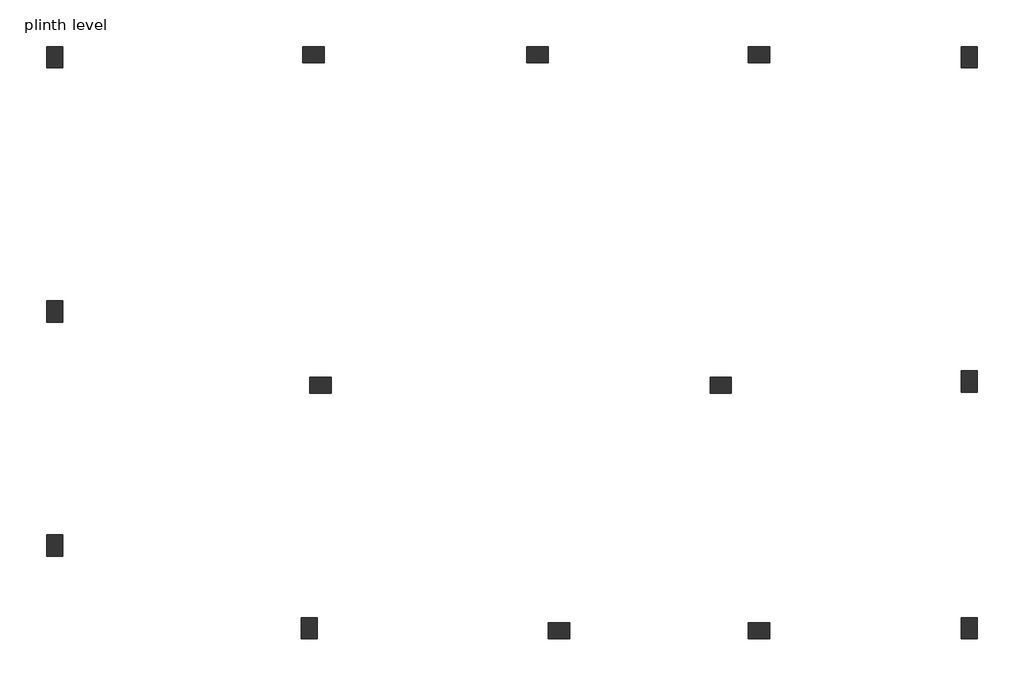
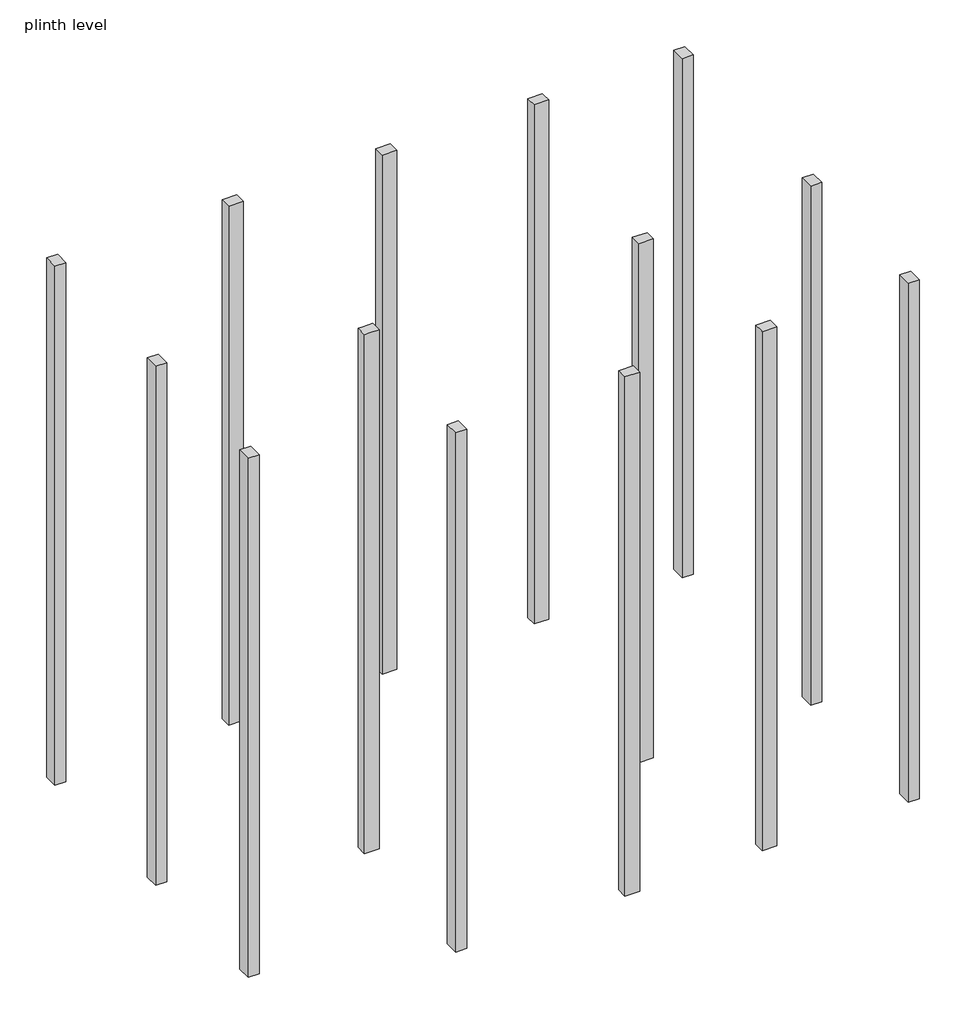
# One storey: 14 columns.
"""IFC4 building model written with IfcOpenShell, lengths in millimetres."""

from ifc_helpers import new_model, si_unit, origin, place, context, project, spatial, faceted_brep, element, save

model = new_model("IFC4")

# Units and contexts
model_context = context("Model", 3, world=origin())
ifc_project = project(units=[si_unit("LENGTHUNIT", "METRE", prefix="MILLI")], contexts=[model_context])

# Site, building, storey
site = spatial("IfcSite", under=ifc_project)
building = spatial("IfcBuilding", under=site)
storey = spatial("IfcBuildingStorey", under=building, Name="plinth level", Elevation=-1219.2)

# Columns
placement = place(None, origin())
element("IfcColumn", 1, ObjectType="Concrete-Rectangular-Column", at=placement, inside=storey, context=model_context, shape_type="Brep", body=[
    faceted_brep([(-8931.9263529, 6682.6661978, -1219.2), (-8931.9263529, 6377.8661978, -1219.2), (-9160.5263529, 6377.8661978, -1219.2), (-9160.5263529, 6682.6661978, -1219.2), (-8931.9263529, 6682.6661978, 10210.8), (-8931.9263529, 6377.8661978, 10210.8), (-8931.9263529, 6377.8661978, 9906.0), (-8931.9263529, 6377.8661978, 7010.4), (-8931.9263529, 6377.8661978, 6705.6), (-8931.9263529, 6377.8661978, 3810.0), (-8931.9263529, 6377.8661978, 3505.2), (-8931.9263529, 6377.8661978, 609.6), (-8931.9263529, 6377.8661978, 304.8), (-8931.9263529, 6682.6661978, 304.8), (-8931.9263529, 6682.6661978, 609.6), (-8931.9263529, 6682.6661978, 3505.2), (-8931.9263529, 6682.6661978, 3810.0), (-8931.9263529, 6682.6661978, 6705.6), (-8931.9263529, 6682.6661978, 7010.4), (-8931.9263529, 6682.6661978, 9906.0), (-9160.5263529, 6377.8661978, 10210.8), (-9160.5263529, 6377.8661978, 9906.0), (-9160.5263529, 6377.8661978, 7010.4), (-9160.5263529, 6377.8661978, 6705.6), (-9160.5263529, 6377.8661978, 3810.0), (-9160.5263529, 6377.8661978, 3505.2), (-9160.5263529, 6377.8661978, 609.6), (-9160.5263529, 6377.8661978, 304.8), (-9160.5263529, 6682.6661978, 10210.8), (-9160.5263529, 6682.6661978, 9906.0), (-9160.5263529, 6682.6661978, 7010.4), (-9160.5263529, 6682.6661978, 6705.6), (-9160.5263529, 6682.6661978, 3810.0), (-9160.5263529, 6682.6661978, 3505.2), (-9160.5263529, 6682.6661978, 609.6), (-9160.5263529, 6682.6661978, 304.8)], [[[0, 1, 2, 3]], [[4, 5, 6, 7, 8, 9, 10, 11, 12, 1, 0, 13, 14, 15, 16, 17, 18, 19]], [[5, 20, 21, 22, 23, 24, 25, 26, 27, 2, 1, 12, 11, 10, 9, 8, 7, 6]], [[20, 28, 29, 30, 31, 32, 33, 34, 35, 3, 2, 27, 26, 25, 24, 23, 22, 21]], [[28, 4, 19, 18, 17, 16, 15, 14, 13, 0, 3, 35, 34, 33, 32, 31, 30, 29]], [[4, 28, 20, 5]]]),
])
element("IfcColumn", 2, ObjectType="Concrete-Rectangular-Column", at=placement, inside=storey, context=model_context, shape_type="Brep", body=[
    faceted_brep([(-5502.9263529, 6682.6661978, -1219.2), (-5198.1263529, 6682.6661978, -1219.2), (-5198.1263529, 6454.0661978, -1219.2), (-5502.9263529, 6454.0661978, -1219.2), (-5502.9263529, 6682.6661978, 10210.8), (-5198.1263529, 6682.6661978, 10210.8), (-5198.1263529, 6644.5661978, 10210.8), (-5198.1263529, 6454.0661978, 10210.8), (-5198.1263529, 6454.0661978, 9906.0), (-5198.1263529, 6454.0661978, 7010.4), (-5198.1263529, 6454.0661978, 6705.6), (-5198.1263529, 6454.0661978, 3810.0), (-5198.1263529, 6454.0661978, 3505.2), (-5198.1263529, 6454.0661978, 609.6), (-5198.1263529, 6454.0661978, 304.8), (-5502.9263529, 6454.0661978, 10210.8), (-5502.9263529, 6454.0661978, 9906.0), (-5502.9263529, 6454.0661978, 7010.4), (-5502.9263529, 6454.0661978, 6705.6), (-5502.9263529, 6454.0661978, 3810.0), (-5502.9263529, 6454.0661978, 3505.2), (-5502.9263529, 6454.0661978, 609.6), (-5502.9263529, 6454.0661978, 304.8), (-5502.9263529, 6644.5661978, 10210.8)], [[[0, 1, 2, 3]], [[4, 5, 1, 0]], [[5, 6, 7, 8, 9, 10, 11, 12, 13, 14, 2, 1]], [[7, 15, 16, 17, 18, 19, 20, 21, 22, 3, 2, 14, 13, 12, 11, 10, 9, 8]], [[15, 23, 4, 0, 3, 22, 21, 20, 19, 18, 17, 16]], [[4, 23, 15, 7, 6, 5]]]),
])
element("IfcColumn", 3, ObjectType="Concrete-Rectangular-Column", at=placement, inside=storey, context=model_context, shape_type="Brep", body=[
    faceted_brep([(-2302.5263529, 6682.6661978, -1219.2), (-1997.7263529, 6682.6661978, -1219.2), (-1997.7263529, 6454.0661978, -1219.2), (-2302.5263529, 6454.0661978, -1219.2), (-2302.5263529, 6682.6661978, 10210.8), (-1997.7263529, 6682.6661978, 10210.8), (-1997.7263529, 6644.5661978, 10210.8), (-1997.7263529, 6454.0661978, 10210.8), (-1997.7263529, 6454.0661978, 9906.0), (-1997.7263529, 6454.0661978, 7010.4), (-1997.7263529, 6454.0661978, 6705.6), (-1997.7263529, 6454.0661978, 3810.0), (-1997.7263529, 6454.0661978, 3505.2), (-1997.7263529, 6454.0661978, 609.6), (-1997.7263529, 6454.0661978, 304.8), (-2302.5263529, 6454.0661978, 10210.8), (-2302.5263529, 6454.0661978, 9906.0), (-2302.5263529, 6454.0661978, 7010.4), (-2302.5263529, 6454.0661978, 6705.6), (-2302.5263529, 6454.0661978, 3810.0), (-2302.5263529, 6454.0661978, 3505.2), (-2302.5263529, 6454.0661978, 609.6), (-2302.5263529, 6454.0661978, 304.8), (-2302.5263529, 6644.5661978, 10210.8)], [[[0, 1, 2, 3]], [[4, 5, 1, 0]], [[5, 6, 7, 8, 9, 10, 11, 12, 13, 14, 2, 1]], [[7, 15, 16, 17, 18, 19, 20, 21, 22, 3, 2, 14, 13, 12, 11, 10, 9, 8]], [[15, 23, 4, 0, 3, 22, 21, 20, 19, 18, 17, 16]], [[4, 23, 15, 7, 6, 5]]]),
])
element("IfcColumn", 4, ObjectType="Concrete-Rectangular-Column", at=placement, inside=storey, context=model_context, shape_type="Brep", body=[
    faceted_brep([(859.7736471, 6682.6661978, -1219.2), (1164.5736471, 6682.6661978, -1219.2), (1164.5736471, 6454.0661978, -1219.2), (859.7736471, 6454.0661978, -1219.2), (859.7736471, 6682.6661978, 10210.8), (1164.5736471, 6682.6661978, 10210.8), (1164.5736471, 6644.5661978, 10210.8), (1164.5736471, 6454.0661978, 10210.8), (1164.5736471, 6454.0661978, 9906.0), (1164.5736471, 6454.0661978, 7010.4), (1164.5736471, 6454.0661978, 6705.6), (1164.5736471, 6454.0661978, 3810.0), (1164.5736471, 6454.0661978, 3505.2), (1164.5736471, 6454.0661978, 609.6), (1164.5736471, 6454.0661978, 304.8), (859.7736471, 6454.0661978, 10210.8), (859.7736471, 6454.0661978, 9906.0), (859.7736471, 6454.0661978, 7010.4), (859.7736471, 6454.0661978, 6705.6), (859.7736471, 6454.0661978, 3810.0), (859.7736471, 6454.0661978, 3505.2), (859.7736471, 6454.0661978, 609.6), (859.7736471, 6454.0661978, 304.8), (859.7736471, 6644.5661978, 10210.8)], [[[0, 1, 2, 3]], [[4, 5, 1, 0]], [[5, 6, 7, 8, 9, 10, 11, 12, 13, 14, 2, 1]], [[7, 15, 16, 17, 18, 19, 20, 21, 22, 3, 2, 14, 13, 12, 11, 10, 9, 8]], [[15, 23, 4, 0, 3, 22, 21, 20, 19, 18, 17, 16]], [[4, 23, 15, 7, 6, 5]]]),
])
element("IfcColumn", 5, ObjectType="Concrete-Rectangular-Column", at=placement, inside=storey, context=model_context, shape_type="Brep", body=[
    faceted_brep([(3901.4236471, 6377.8661978, -1219.2), (3901.4236471, 6682.6661978, -1219.2), (4130.0236471, 6682.6661978, -1219.2), (4130.0236471, 6377.8661978, -1219.2), (3901.4236471, 6377.8661978, 10210.8), (3901.4236471, 6682.6661978, 10210.8), (3901.4236471, 6377.8661978, 304.8), (3901.4236471, 6377.8661978, 609.6), (4130.0236471, 6682.6661978, 10210.8), (4130.0236471, 6377.8661978, 10210.8), (4130.0236471, 6377.8661978, 609.6), (4130.0236471, 6377.8661978, 304.8)], [[[0, 1, 2, 3]], [[4, 5, 1, 0, 6, 7]], [[5, 8, 2, 1]], [[8, 9, 10, 11, 3, 2]], [[9, 4, 7, 6, 0, 3, 11, 10]], [[4, 9, 8, 5]]]),
])
element("IfcColumn", 6, ObjectType="Concrete-Rectangular-Column", at=placement, inside=storey, context=model_context, shape_type="Brep", body=[
    faceted_brep([(3901.4236471, 1748.7161978, -1219.2), (3901.4236471, 2053.5161978, -1219.2), (4130.0236471, 2053.5161978, -1219.2), (4130.0236471, 1748.7161978, -1219.2), (3901.4236471, 1748.7161978, 10210.8), (3901.4236471, 2053.5161978, 10210.8), (3901.4236471, 2053.5161978, 9906.0), (3901.4236471, 2053.5161978, 7010.4), (3901.4236471, 2053.5161978, 6705.6), (3901.4236471, 2053.5161978, 3810.0), (3901.4236471, 2053.5161978, 3505.2), (3901.4236471, 2053.5161978, 609.6), (3901.4236471, 2053.5161978, 304.8), (3901.4236471, 1748.7161978, 304.8), (3901.4236471, 1748.7161978, 609.6), (3901.4236471, 1748.7161978, 3505.2), (3901.4236471, 1748.7161978, 3810.0), (3901.4236471, 1748.7161978, 6705.6), (3901.4236471, 1748.7161978, 7010.4), (3901.4236471, 1748.7161978, 9906.0), (4130.0236471, 2053.5161978, 10210.8), (4130.0236471, 2053.5161978, 9906.0), (4130.0236471, 2053.5161978, 7010.4), (4130.0236471, 2053.5161978, 6705.6), (4130.0236471, 2053.5161978, 3810.0), (4130.0236471, 2053.5161978, 3505.2), (4130.0236471, 2053.5161978, 609.6), (4130.0236471, 2053.5161978, 304.8), (4130.0236471, 1748.7161978, 10210.8), (4130.0236471, 1748.7161978, 9906.0), (4130.0236471, 1748.7161978, 7010.4), (4130.0236471, 1748.7161978, 6705.6), (4130.0236471, 1748.7161978, 3810.0), (4130.0236471, 1748.7161978, 3505.2), (4130.0236471, 1748.7161978, 609.6), (4130.0236471, 1748.7161978, 304.8)], [[[0, 1, 2, 3]], [[4, 5, 6, 7, 8, 9, 10, 11, 12, 1, 0, 13, 14, 15, 16, 17, 18, 19]], [[5, 20, 21, 22, 23, 24, 25, 26, 27, 2, 1, 12, 11, 10, 9, 8, 7, 6]], [[20, 28, 29, 30, 31, 32, 33, 34, 35, 3, 2, 27, 26, 25, 24, 23, 22, 21]], [[28, 4, 19, 18, 17, 16, 15, 14, 13, 0, 3, 35, 34, 33, 32, 31, 30, 29]], [[4, 28, 20, 5]]]),
])
element("IfcColumn", 7, ObjectType="Concrete-Rectangular-Column", at=placement, inside=storey, context=model_context, shape_type="Brep", body=[
    faceted_brep([(3901.4236471, -1775.5338022, -1219.2), (3901.4236471, -1470.7338022, -1219.2), (4130.0236471, -1470.7338022, -1219.2), (4130.0236471, -1775.5338022, -1219.2), (3901.4236471, -1775.5338022, 10210.8), (3901.4236471, -1470.7338022, 10210.8), (3901.4236471, -1470.7338022, 609.6), (3901.4236471, -1470.7338022, 304.8), (4130.0236471, -1470.7338022, 10210.8), (4130.0236471, -1470.7338022, 609.6), (4130.0236471, -1470.7338022, 304.8), (4130.0236471, -1775.5338022, 10210.8)], [[[0, 1, 2, 3]], [[4, 5, 6, 7, 1, 0]], [[5, 8, 9, 10, 2, 1, 7, 6]], [[8, 11, 3, 2, 10, 9]], [[11, 4, 0, 3]], [[4, 11, 8, 5]]]),
])
element("IfcColumn", 8, ObjectType="Concrete-Rectangular-Column", at=placement, inside=storey, context=model_context, shape_type="Brep", body=[
    faceted_brep([(1164.5736471, -1775.5338022, -1219.2), (859.7736471, -1775.5338022, -1219.2), (859.7736471, -1546.9338022, -1219.2), (1164.5736471, -1546.9338022, -1219.2), (1164.5736471, -1775.5338022, 10210.8), (859.7736471, -1775.5338022, 10210.8), (859.7736471, -1737.4338022, 10210.8), (859.7736471, -1546.9338022, 10210.8), (859.7736471, -1546.9338022, 9906.0), (859.7736471, -1546.9338022, 7010.4), (859.7736471, -1546.9338022, 6705.6), (859.7736471, -1546.9338022, 3810.0), (859.7736471, -1546.9338022, 3505.2), (859.7736471, -1546.9338022, 609.6), (859.7736471, -1546.9338022, 304.8), (1164.5736471, -1546.9338022, 10210.8), (1164.5736471, -1546.9338022, 9906.0), (1164.5736471, -1546.9338022, 7010.4), (1164.5736471, -1546.9338022, 6705.6), (1164.5736471, -1546.9338022, 3810.0), (1164.5736471, -1546.9338022, 3505.2), (1164.5736471, -1546.9338022, 609.6), (1164.5736471, -1546.9338022, 304.8), (1164.5736471, -1737.4338022, 10210.8)], [[[0, 1, 2, 3]], [[4, 5, 1, 0]], [[5, 6, 7, 8, 9, 10, 11, 12, 13, 14, 2, 1]], [[7, 15, 16, 17, 18, 19, 20, 21, 22, 3, 2, 14, 13, 12, 11, 10, 9, 8]], [[15, 23, 4, 0, 3, 22, 21, 20, 19, 18, 17, 16]], [[4, 23, 15, 7, 6, 5]]]),
])
element("IfcColumn", 9, ObjectType="Concrete-Rectangular-Column", at=placement, inside=storey, context=model_context, shape_type="Brep", body=[
    faceted_brep([(-1692.9263529, -1775.5338022, -1219.2), (-1997.7263529, -1775.5338022, -1219.2), (-1997.7263529, -1546.9338022, -1219.2), (-1692.9263529, -1546.9338022, -1219.2), (-1692.9263529, -1775.5338022, 10210.8), (-1997.7263529, -1775.5338022, 10210.8), (-1997.7263529, -1737.4338022, 10210.8), (-1997.7263529, -1546.9338022, 10210.8), (-1997.7263529, -1546.9338022, 9906.0), (-1997.7263529, -1546.9338022, 7010.4), (-1997.7263529, -1546.9338022, 6705.6), (-1997.7263529, -1546.9338022, 3810.0), (-1997.7263529, -1546.9338022, 3505.2), (-1997.7263529, -1546.9338022, 609.6), (-1997.7263529, -1546.9338022, 304.8), (-1692.9263529, -1546.9338022, 10210.8), (-1692.9263529, -1546.9338022, 9906.0), (-1692.9263529, -1546.9338022, 7010.4), (-1692.9263529, -1546.9338022, 6705.6), (-1692.9263529, -1546.9338022, 3810.0), (-1692.9263529, -1546.9338022, 3505.2), (-1692.9263529, -1546.9338022, 609.6), (-1692.9263529, -1546.9338022, 304.8), (-1692.9263529, -1737.4338022, 10210.8)], [[[0, 1, 2, 3]], [[4, 5, 1, 0]], [[5, 6, 7, 8, 9, 10, 11, 12, 13, 14, 2, 1]], [[7, 15, 16, 17, 18, 19, 20, 21, 22, 3, 2, 14, 13, 12, 11, 10, 9, 8]], [[15, 23, 4, 0, 3, 22, 21, 20, 19, 18, 17, 16]], [[4, 23, 15, 7, 6, 5]]]),
])
element("IfcColumn", 10, ObjectType="Concrete-Rectangular-Column", at=placement, inside=storey, context=model_context, shape_type="Brep", body=[
    faceted_brep([(-5293.3763529, -1470.7338022, -1219.2), (-5293.3763529, -1775.5338022, -1219.2), (-5521.9763529, -1775.5338022, -1219.2), (-5521.9763529, -1470.7338022, -1219.2), (-5293.3763529, -1470.7338022, 10210.8), (-5293.3763529, -1775.5338022, 10210.8), (-5293.3763529, -1470.7338022, 304.8), (-5293.3763529, -1470.7338022, 609.6), (-5521.9763529, -1775.5338022, 10210.8), (-5521.9763529, -1470.7338022, 10210.8), (-5521.9763529, -1470.7338022, 609.6), (-5521.9763529, -1470.7338022, 304.8)], [[[0, 1, 2, 3]], [[4, 5, 1, 0, 6, 7]], [[5, 8, 2, 1]], [[8, 9, 10, 11, 3, 2]], [[9, 4, 7, 6, 0, 3, 11, 10]], [[4, 9, 8, 5]]]),
])
element("IfcColumn", 11, ObjectType="Concrete-Rectangular-Column", at=placement, inside=storey, context=model_context, shape_type="Brep", body=[
    faceted_brep([(-8931.9263529, -289.6338022, -1219.2), (-8931.9263529, -594.4338022, -1219.2), (-9160.5263529, -594.4338022, -1219.2), (-9160.5263529, -289.6338022, -1219.2), (-8931.9263529, -289.6338022, 10210.8), (-8931.9263529, -594.4338022, 10210.8), (-8931.9263529, -289.6338022, 304.8), (-8931.9263529, -289.6338022, 609.6), (-9160.5263529, -594.4338022, 10210.8), (-9160.5263529, -289.6338022, 10210.8), (-9160.5263529, -289.6338022, 609.6), (-9160.5263529, -289.6338022, 304.8)], [[[0, 1, 2, 3]], [[4, 5, 1, 0, 6, 7]], [[5, 8, 2, 1]], [[8, 9, 10, 11, 3, 2]], [[9, 4, 7, 6, 0, 3, 11, 10]], [[4, 9, 8, 5]]]),
])
element("IfcColumn", 12, ObjectType="Concrete-Rectangular-Column", at=placement, inside=storey, context=model_context, shape_type="Brep", body=[
    faceted_brep([(-8931.9263529, 3050.4661978, -1219.2), (-8931.9263529, 2745.6661978, -1219.2), (-9160.5263529, 2745.6661978, -1219.2), (-9160.5263529, 3050.4661978, -1219.2), (-8931.9263529, 3050.4661978, 10210.8), (-8931.9263529, 2745.6661978, 10210.8), (-8931.9263529, 2745.6661978, 9906.0), (-8931.9263529, 2745.6661978, 7010.4), (-8931.9263529, 2745.6661978, 6705.6), (-8931.9263529, 2745.6661978, 3810.0), (-8931.9263529, 2745.6661978, 3505.2), (-8931.9263529, 2745.6661978, 609.6), (-8931.9263529, 2745.6661978, 304.8), (-8931.9263529, 3050.4661978, 304.8), (-8931.9263529, 3050.4661978, 609.6), (-8931.9263529, 3050.4661978, 3505.2), (-8931.9263529, 3050.4661978, 3810.0), (-8931.9263529, 3050.4661978, 6705.6), (-8931.9263529, 3050.4661978, 7010.4), (-8931.9263529, 3050.4661978, 9906.0), (-9160.5263529, 2745.6661978, 10210.8), (-9160.5263529, 2745.6661978, 9906.0), (-9160.5263529, 2745.6661978, 7010.4), (-9160.5263529, 2745.6661978, 6705.6), (-9160.5263529, 2745.6661978, 3810.0), (-9160.5263529, 2745.6661978, 3505.2), (-9160.5263529, 2745.6661978, 609.6), (-9160.5263529, 2745.6661978, 304.8), (-9160.5263529, 3050.4661978, 10210.8), (-9160.5263529, 3050.4661978, 9906.0), (-9160.5263529, 3050.4661978, 7010.4), (-9160.5263529, 3050.4661978, 6705.6), (-9160.5263529, 3050.4661978, 3810.0), (-9160.5263529, 3050.4661978, 3505.2), (-9160.5263529, 3050.4661978, 609.6), (-9160.5263529, 3050.4661978, 304.8)], [[[0, 1, 2, 3]], [[4, 5, 6, 7, 8, 9, 10, 11, 12, 1, 0, 13, 14, 15, 16, 17, 18, 19]], [[5, 20, 21, 22, 23, 24, 25, 26, 27, 2, 1, 12, 11, 10, 9, 8, 7, 6]], [[20, 28, 29, 30, 31, 32, 33, 34, 35, 3, 2, 27, 26, 25, 24, 23, 22, 21]], [[28, 4, 19, 18, 17, 16, 15, 14, 13, 0, 3, 35, 34, 33, 32, 31, 30, 29]], [[4, 28, 20, 5]]]),
])
element("IfcColumn", 13, ObjectType="Concrete-Rectangular-Column", at=placement, inside=storey, context=model_context, shape_type="Brep", body=[
    faceted_brep([(-5401.3263529, 1958.2661978, -1219.2), (-5096.5263529, 1958.2661978, -1219.2), (-5096.5263529, 1729.6661978, -1219.2), (-5401.3263529, 1729.6661978, -1219.2), (-5401.3263529, 1958.2661978, 10210.8), (-5293.3763529, 1958.2661978, 10210.8), (-5096.5263529, 1958.2661978, 10210.8), (-5096.5263529, 1958.2661978, 9906.0), (-5096.5263529, 1958.2661978, 7010.4), (-5096.5263529, 1958.2661978, 6705.6), (-5096.5263529, 1958.2661978, 3810.0), (-5096.5263529, 1958.2661978, 3505.2), (-5096.5263529, 1958.2661978, 609.6), (-5096.5263529, 1958.2661978, 304.8), (-5401.3263529, 1958.2661978, 304.8), (-5401.3263529, 1958.2661978, 609.6), (-5401.3263529, 1958.2661978, 3505.2), (-5401.3263529, 1958.2661978, 3810.0), (-5401.3263529, 1958.2661978, 6705.6), (-5401.3263529, 1958.2661978, 7010.4), (-5401.3263529, 1958.2661978, 9906.0), (-5096.5263529, 1729.6661978, 10210.8), (-5096.5263529, 1729.6661978, 9906.0), (-5096.5263529, 1729.6661978, 7010.4), (-5096.5263529, 1729.6661978, 6705.6), (-5096.5263529, 1729.6661978, 3810.0), (-5096.5263529, 1729.6661978, 3505.2), (-5096.5263529, 1729.6661978, 609.6), (-5096.5263529, 1729.6661978, 304.8), (-5293.3763529, 1729.6661978, 10210.8), (-5401.3263529, 1729.6661978, 10210.8), (-5401.3263529, 1729.6661978, 9906.0), (-5401.3263529, 1729.6661978, 7010.4), (-5401.3263529, 1729.6661978, 6705.6), (-5401.3263529, 1729.6661978, 3810.0), (-5401.3263529, 1729.6661978, 3505.2), (-5401.3263529, 1729.6661978, 609.6), (-5401.3263529, 1729.6661978, 304.8)], [[[0, 1, 2, 3]], [[4, 5, 6, 7, 8, 9, 10, 11, 12, 13, 1, 0, 14, 15, 16, 17, 18, 19, 20]], [[6, 21, 22, 23, 24, 25, 26, 27, 28, 2, 1, 13, 12, 11, 10, 9, 8, 7]], [[21, 29, 30, 31, 32, 33, 34, 35, 36, 37, 3, 2, 28, 27, 26, 25, 24, 23, 22]], [[30, 4, 20, 19, 18, 17, 16, 15, 14, 0, 3, 37, 36, 35, 34, 33, 32, 31]], [[4, 30, 29, 21, 6, 5]]]),
])
element("IfcColumn", 14, ObjectType="Concrete-Rectangular-Column", at=placement, inside=storey, context=model_context, shape_type="Brep", body=[
    faceted_brep([(313.6736471, 1958.2661978, -1219.2), (618.4736471, 1958.2661978, -1219.2), (618.4736471, 1729.6661978, -1219.2), (313.6736471, 1729.6661978, -1219.2), (313.6736471, 1958.2661978, 10210.8), (618.4736471, 1958.2661978, 10210.8), (618.4736471, 1958.2661978, 9906.0), (618.4736471, 1958.2661978, 7010.4), (618.4736471, 1958.2661978, 6705.6), (618.4736471, 1958.2661978, 3810.0), (618.4736471, 1958.2661978, 3505.2), (618.4736471, 1958.2661978, 609.6), (618.4736471, 1958.2661978, 304.8), (313.6736471, 1958.2661978, 304.8), (313.6736471, 1958.2661978, 609.6), (313.6736471, 1958.2661978, 3505.2), (313.6736471, 1958.2661978, 3810.0), (313.6736471, 1958.2661978, 6705.6), (313.6736471, 1958.2661978, 7010.4), (313.6736471, 1958.2661978, 9906.0), (618.4736471, 1729.6661978, 10210.8), (618.4736471, 1729.6661978, 9906.0), (618.4736471, 1729.6661978, 7010.4), (618.4736471, 1729.6661978, 6705.6), (618.4736471, 1729.6661978, 3810.0), (618.4736471, 1729.6661978, 3505.2), (618.4736471, 1729.6661978, 609.6), (618.4736471, 1729.6661978, 304.8), (313.6736471, 1729.6661978, 10210.8), (313.6736471, 1729.6661978, 9906.0), (313.6736471, 1729.6661978, 7010.4), (313.6736471, 1729.6661978, 6705.6), (313.6736471, 1729.6661978, 3810.0), (313.6736471, 1729.6661978, 3505.2), (313.6736471, 1729.6661978, 609.6), (313.6736471, 1729.6661978, 304.8)], [[[0, 1, 2, 3]], [[4, 5, 6, 7, 8, 9, 10, 11, 12, 1, 0, 13, 14, 15, 16, 17, 18, 19]], [[5, 20, 21, 22, 23, 24, 25, 26, 27, 2, 1, 12, 11, 10, 9, 8, 7, 6]], [[20, 28, 29, 30, 31, 32, 33, 34, 35, 3, 2, 27, 26, 25, 24, 23, 22, 21]], [[28, 4, 19, 18, 17, 16, 15, 14, 13, 0, 3, 35, 34, 33, 32, 31, 30, 29]], [[4, 28, 20, 5]]]),
])

save(model, "model.ifc")

# Revit data of these elements
# Type "Concrete-Rectangular-Column"
#   Assembly Code = "B10"
#   b = 0' - 9"
#   h = 1' - 0"
#   Structural Material [instance default] = Concrete, Cast-in-Place gray
# Elements 1, 2, 3, 4, 5, 6, 7, 8, 9, 10, 11, 12, 13, 14 (IfcColumn, "Concrete-Rectangular-Column")
#   Structural Material = Concrete, Cast-in-Place gray
#   Phase Created = New Construction
#   Materials on its faces: "Concrete, Cast-in-Place gray"
# Materials
#   "Concrete, Cast-in-Place gray": class "Concrete", colour RGB 192 192 192, transparency 0, Description = "Cast-in-place concrete", Cost = 0
